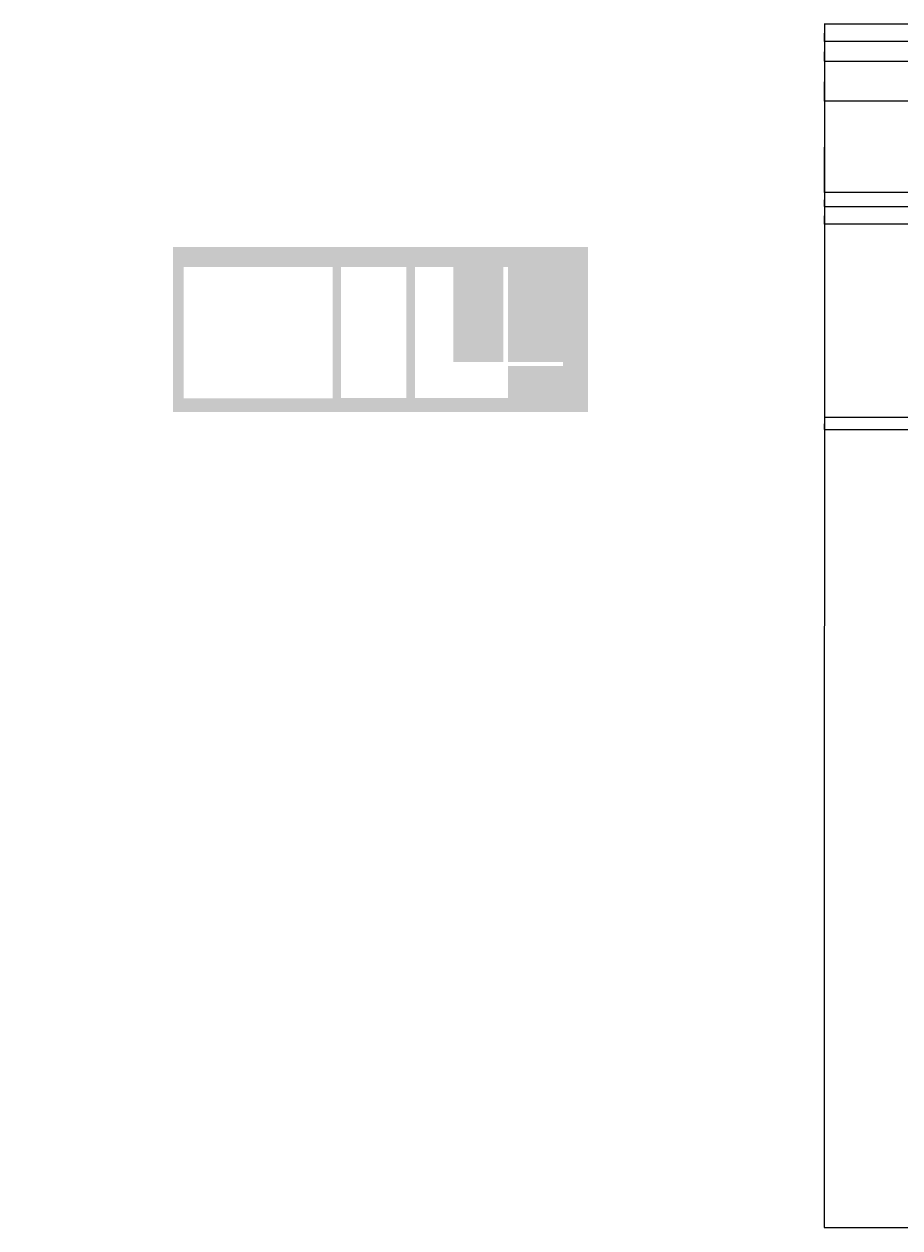
# Model space of a CAD drawing. Units: feet. Extents: x 1141 to 2858, y 751 to 1654.
# Tile 1 of 13: x 1141 to 1718, y 806 to 1599. Entities that reach past the tile are written whole.
import ezdxf

# ---------------------------------------------------------------- set-up
doc = ezdxf.new("R2010")
doc.units = ezdxf.units.FT
doc.layers.add('A-ANNO-DIMS', color=2, linetype='Continuous', lineweight=18)
doc.layers.add('A-ELEV-PATT', color=8, linetype='Continuous', lineweight=13)
doc.styles.get("Standard").update_dxf_attribs({"font": 'arial.ttf'})
doc.dimstyles.get("Standard").update_dxf_attribs({"dimtxt": 0.18, "dimasz": 0.18, "dimexe": 0.18, "dimexo": 0.0625, "dimgap": 0.09, "dimtad": 0, "dimtih": 1, "dimtoh": 1, "dimdec": 1, "dimzin": 0, "dimdsep": 46, "dimlunit": 3, "dimtxsty": 'Standard', "dimcen": 0.09, "dimadec": 0, "dimazin": 0, "dimtfac": 1, "dimtdec": 1, "dimtofl": 0, "dimtmove": 0, "dimatfit": 3, "dimfxl": 1, "dimtolj": 1, "dimtzin": 0, "dimarcsym": 0})

# ---------------------------------------------------------------- blocks, each defined once
blk = doc.blocks.new('*D24')
at = {"layer": 'A-ANNO-DIMS', "color": 0, "lineweight": -2, "transparency": 16777216}
for p, q in [((1725.97, 1599.45), (1668.14, 1599.45)), ((1668.32, 1599.27), (1668.32, 1202.86)), ((1668.32, 806.08), (1668.32, 1202.49)), ((1725.97, 805.9), (1668.14, 805.9))]:
    blk.add_line(p, q, dxfattribs=at)
at = {"layer": 'A-ANNO-DIMS', "color": 0, "transparency": 16777216}
for points in [[(1668.29, 1599.27), (1668.35, 1599.27), (1668.32, 1599.45)], [(1668.29, 806.08), (1668.35, 806.08), (1668.32, 805.9)]]:
    blk.add_solid(points, dxfattribs=at)
at = {"layer": 'Defpoints', "color": 0, "transparency": 16777216}
for p in [(1668.32, 1599.45), (1726.03, 1599.45), (1726.03, 805.9)]:
    blk.add_point(p, dxfattribs=at)
at = {"layer": 'A-ANNO-DIMS', "color": 0, "transparency": 16777216, "insert": (1668.32, 1202.68), "char_height": 0.18, "attachment_point": 5}
blk.add_mtext('\\A1;793.6', dxfattribs=at)
blk = doc.blocks.new('*D39')
at = {"layer": 'A-ANNO-DIMS', "color": 0, "lineweight": -2, "transparency": 16777216}
for p, q in [((2319.24, 1599.45), (1668.14, 1599.45)), ((1668.32, 1599.27), (1668.32, 1202.86)), ((1668.32, 806.08), (1668.32, 1202.49)), ((2319.24, 805.9), (1668.14, 805.9))]:
    blk.add_line(p, q, dxfattribs=at)
at = {"layer": 'A-ANNO-DIMS', "color": 0, "transparency": 16777216}
for points in [[(1668.29, 1599.27), (1668.35, 1599.27), (1668.32, 1599.45)], [(1668.29, 806.08), (1668.35, 806.08), (1668.32, 805.9)]]:
    blk.add_solid(points, dxfattribs=at)
at = {"layer": 'Defpoints', "color": 0, "transparency": 16777216}
for p in [(1668.32, 1599.45), (2319.3, 1599.45), (2319.3, 805.9)]:
    blk.add_point(p, dxfattribs=at)
at = {"layer": 'A-ANNO-DIMS', "color": 0, "transparency": 16777216, "insert": (1668.32, 1202.68), "char_height": 0.18, "attachment_point": 5}
blk.add_mtext('\\A1;793.6', dxfattribs=at)
blk = doc.blocks.new('*D48')
at = {"layer": 'A-ANNO-DIMS', "color": 0, "lineweight": -2, "transparency": 16777216}
for p, q in [((2330.82, 1479.03), (1668.14, 1479.03)), ((1668.32, 1478.85), (1668.32, 1473.42)), ((1668.32, 1467.63), (1668.32, 1473.06)), ((2319.24, 1467.45), (1668.14, 1467.45))]:
    blk.add_line(p, q, dxfattribs=at)
at = {"layer": 'A-ANNO-DIMS', "color": 0, "transparency": 16777216}
for points in [[(1668.29, 1478.85), (1668.35, 1478.85), (1668.32, 1479.03)], [(1668.29, 1467.63), (1668.35, 1467.63), (1668.32, 1467.45)]]:
    blk.add_solid(points, dxfattribs=at)
at = {"layer": 'Defpoints', "color": 0, "transparency": 16777216}
for p in [(1668.32, 1479.03), (2330.88, 1479.03), (2319.3, 1467.45)]:
    blk.add_point(p, dxfattribs=at)
at = {"layer": 'A-ANNO-DIMS', "color": 0, "transparency": 16777216, "insert": (1668.32, 1473.24), "char_height": 0.18, "attachment_point": 5}
blk.add_mtext('\\A1;11.58', dxfattribs=at)
blk = doc.blocks.new('*D49')
at = {"layer": 'A-ANNO-DIMS', "color": 0, "lineweight": -2, "transparency": 16777216}
for p, q in [((2347.45, 1488.33), (1668.14, 1488.33)), ((1668.32, 1488.15), (1668.32, 1483.86)), ((2330.82, 1479.03), (1668.14, 1479.03)), ((1668.32, 1479.21), (1668.32, 1483.5))]:
    blk.add_line(p, q, dxfattribs=at)
at = {"layer": 'A-ANNO-DIMS', "color": 0, "transparency": 16777216}
for points in [[(1668.29, 1488.15), (1668.35, 1488.15), (1668.32, 1488.33)], [(1668.29, 1479.21), (1668.35, 1479.21), (1668.32, 1479.03)]]:
    blk.add_solid(points, dxfattribs=at)
at = {"layer": 'Defpoints', "color": 0, "transparency": 16777216}
for p in [(1668.32, 1488.33), (2347.51, 1488.33), (2330.88, 1479.03)]:
    blk.add_point(p, dxfattribs=at)
at = {"layer": 'A-ANNO-DIMS', "color": 0, "transparency": 16777216, "insert": (1668.32, 1483.68), "char_height": 0.18, "attachment_point": 5}
blk.add_mtext('\\A1;9.293', dxfattribs=at)
blk = doc.blocks.new('*D50')
at = {"layer": 'A-ANNO-DIMS', "color": 0, "lineweight": -2, "transparency": 16777216}
for p, q in [((2356.58, 1548.54), (1668.14, 1548.54)), ((1668.32, 1548.36), (1668.32, 1518.62)), ((1668.32, 1488.51), (1668.32, 1518.25)), ((2347.45, 1488.33), (1668.14, 1488.33))]:
    blk.add_line(p, q, dxfattribs=at)
at = {"layer": 'A-ANNO-DIMS', "color": 0, "transparency": 16777216}
for points in [[(1668.29, 1548.36), (1668.35, 1548.36), (1668.32, 1548.54)], [(1668.29, 1488.51), (1668.35, 1488.51), (1668.32, 1488.33)]]:
    blk.add_solid(points, dxfattribs=at)
at = {"layer": 'Defpoints', "color": 0, "transparency": 16777216}
for p in [(1668.32, 1548.54), (2356.64, 1548.54), (2347.51, 1488.33)]:
    blk.add_point(p, dxfattribs=at)
at = {"layer": 'A-ANNO-DIMS', "color": 0, "transparency": 16777216, "insert": (1668.32, 1518.43), "char_height": 0.18, "attachment_point": 5}
blk.add_mtext('\\A1;60.22', dxfattribs=at)
blk = doc.blocks.new('*D51')
at = {"layer": 'A-ANNO-DIMS', "color": 0, "lineweight": -2, "transparency": 16777216}
for p, q in [((2347.45, 1574.77), (1668.14, 1574.77)), ((1668.32, 1574.59), (1668.32, 1561.84)), ((1668.32, 1548.72), (1668.32, 1561.47)), ((2356.58, 1548.54), (1668.14, 1548.54))]:
    blk.add_line(p, q, dxfattribs=at)
at = {"layer": 'A-ANNO-DIMS', "color": 0, "transparency": 16777216}
for points in [[(1668.29, 1574.59), (1668.35, 1574.59), (1668.32, 1574.77)], [(1668.29, 1548.72), (1668.35, 1548.72), (1668.32, 1548.54)]]:
    blk.add_solid(points, dxfattribs=at)
at = {"layer": 'Defpoints', "color": 0, "transparency": 16777216}
for p in [(1668.32, 1574.77), (2347.51, 1574.77), (2356.64, 1548.54)]:
    blk.add_point(p, dxfattribs=at)
at = {"layer": 'A-ANNO-DIMS', "color": 0, "transparency": 16777216, "insert": (1668.32, 1561.66), "char_height": 0.18, "attachment_point": 5}
blk.add_mtext('\\A1;26.23', dxfattribs=at)
blk = doc.blocks.new('*D52')
at = {"layer": 'A-ANNO-DIMS', "color": 0, "lineweight": -2, "transparency": 16777216}
for p, q in [((2330.82, 1587.87), (1668.14, 1587.87)), ((1668.32, 1587.69), (1668.32, 1581.5)), ((1668.32, 1574.95), (1668.32, 1581.14)), ((2347.45, 1574.77), (1668.14, 1574.77))]:
    blk.add_line(p, q, dxfattribs=at)
at = {"layer": 'A-ANNO-DIMS', "color": 0, "transparency": 16777216}
for points in [[(1668.29, 1587.69), (1668.35, 1587.69), (1668.32, 1587.87)], [(1668.29, 1574.95), (1668.35, 1574.95), (1668.32, 1574.77)]]:
    blk.add_solid(points, dxfattribs=at)
at = {"layer": 'Defpoints', "color": 0, "transparency": 16777216}
for p in [(1668.32, 1587.87), (2330.88, 1587.87), (2347.51, 1574.77)]:
    blk.add_point(p, dxfattribs=at)
at = {"layer": 'A-ANNO-DIMS', "color": 0, "transparency": 16777216, "insert": (1668.32, 1581.32), "char_height": 0.18, "attachment_point": 5}
blk.add_mtext('\\A1;13.102', dxfattribs=at)
blk = doc.blocks.new('*D53')
at = {"layer": 'A-ANNO-DIMS', "color": 0, "lineweight": -2, "transparency": 16777216}
for p, q in [((2319.24, 1599.45), (1668.14, 1599.45)), ((1668.32, 1599.27), (1668.32, 1593.84)), ((2330.82, 1587.87), (1668.14, 1587.87)), ((1668.32, 1588.05), (1668.32, 1593.48))]:
    blk.add_line(p, q, dxfattribs=at)
at = {"layer": 'A-ANNO-DIMS', "color": 0, "transparency": 16777216}
for points in [[(1668.29, 1599.27), (1668.35, 1599.27), (1668.32, 1599.45)], [(1668.29, 1588.05), (1668.35, 1588.05), (1668.32, 1587.87)]]:
    blk.add_solid(points, dxfattribs=at)
at = {"layer": 'Defpoints', "color": 0, "transparency": 16777216}
for p in [(1668.32, 1599.45), (2319.3, 1599.45), (2330.88, 1587.87)]:
    blk.add_point(p, dxfattribs=at)
at = {"layer": 'A-ANNO-DIMS', "color": 0, "transparency": 16777216, "insert": (1668.32, 1593.66), "char_height": 0.18, "attachment_point": 5}
blk.add_mtext('\\A1;11.58', dxfattribs=at)
blk = doc.blocks.new('*D54')
at = {"layer": 'A-ANNO-DIMS', "color": 0, "lineweight": -2, "transparency": 16777216}
for p, q in [((2327.22, 1340.05), (1668.14, 1340.05)), ((1668.32, 1339.87), (1668.32, 1336.24)), ((1668.32, 1332.24), (1668.32, 1335.88)), ((2319.24, 1332.06), (1668.14, 1332.06))]:
    blk.add_line(p, q, dxfattribs=at)
at = {"layer": 'A-ANNO-DIMS', "color": 0, "transparency": 16777216}
for points in [[(1668.29, 1339.87), (1668.35, 1339.87), (1668.32, 1340.05)], [(1668.29, 1332.24), (1668.35, 1332.24), (1668.32, 1332.06)]]:
    blk.add_solid(points, dxfattribs=at)
at = {"layer": 'Defpoints', "color": 0, "transparency": 16777216}
for p in [(1668.32, 1340.05), (2327.29, 1340.05), (2319.3, 1332.06)]:
    blk.add_point(p, dxfattribs=at)
at = {"layer": 'A-ANNO-DIMS', "color": 0, "transparency": 16777216, "insert": (1668.32, 1336.06), "char_height": 0.18, "attachment_point": 5}
blk.add_mtext('\\A1;7.986', dxfattribs=at)

msp = doc.modelspace()

# ---------------------------------------------------------------- hatches: boundary and pattern name
at = {"layer": 'A-ELEV-PATT'}
h = msp.add_hatch(color=256, dxfattribs=at)
h.dxf.hatch_style = 1
h.paths.add_polyline_path([(1219.3173, 1456.0789), (1140.7487, 1456.0789), (1156.2318, 1444.9949), (1219.3173, 1444.9949)], flags=0)
h.paths.add_polyline_path([(1156.2318, 1444.9949), (1140.7487, 1456.0789), (1140.7487, 1340.0506), (1156.2318, 1340.0506)], flags=0)
h.paths.add_polyline_path([(1156.2318, 1309.6069), (1187.7746, 1309.6069), (1187.7746, 1242.2735), (1219.3173, 1242.2735), (1219.3173, 1241.454), (1187.7746, 1241.454), (1187.7746, 1204.6626), (1186.8597, 1204.6626), (1186.8597, 1241.454), (1156.2318, 1241.454), (1156.2318, 1242.2735)], flags=0)
h.paths.add_polyline_path([(2109.4211, 1049.9149), (2030.8524, 1049.9149), (2030.8524, 1038.831), (2093.938, 1038.831), (2093.938, 933.8867), (2109.4211, 933.8867)], flags=0)
h.paths.add_polyline_path([(2109.4211, 1185.3029), (2030.8524, 1185.3029), (2030.8524, 1174.219), (2093.938, 1174.219), (2093.938, 1069.2747), (2109.4211, 1069.2747)])
h.paths.add_polyline_path([(1812.5866, 1320.6909), (1734.0179, 1320.6909), (1749.501, 1309.6069), (1812.5866, 1309.6069)])
h.paths.add_polyline_path([(1749.501, 1309.6069), (1734.0179, 1320.6909), (1734.0179, 1204.6626), (1749.501, 1204.6626)])
h.paths.add_polyline_path([(1812.5866, 1456.0789), (1734.0179, 1456.0789), (1749.501, 1444.9949), (1812.5866, 1444.9949)])
h.paths.add_polyline_path([(2117.407, 1057.9008), (2022.8666, 1057.9008), (2022.8666, 925.9008), (2117.407, 925.9008)])
h.paths.add_polyline_path([(2030.8524, 933.8867), (2030.8524, 1049.9149), (2109.4211, 1049.9149), (2109.4211, 933.8867)], flags=16)
h.paths.add_polyline_path([(2062.3952, 933.8867), (2062.3952, 970.6781), (2030.8524, 970.6781), (2030.8524, 971.4975), (2062.3952, 971.4975), (2062.3952, 1038.831), (2063.3101, 1038.831), (2093.938, 1038.831), (2093.938, 970.6781), (2063.3101, 970.6781), (2063.3101, 933.8867)], flags=0)
h = msp.add_hatch(color=256, dxfattribs=at)
h.dxf.hatch_style = 1
h.paths.add_polyline_path([(1512.5575, 1452.4845), (1238.8835, 1452.4845), (1238.8835, 1343.645), (1245.9375, 1352.9376), (1245.9375, 1439.3822), (1344.0874, 1439.3822), (1344.0874, 1352.9376), (1349.6277, 1352.9376), (1349.6277, 1439.3822), (1392.6132, 1439.3822), (1392.6132, 1352.9376), (1398.5284, 1352.9376), (1398.5284, 1439.3822), (1423.6034, 1439.3822), (1423.6034, 1376.6436), (1456.7296, 1376.6436), (1456.7296, 1439.3822), (1459.7654, 1439.3822), (1459.7654, 1376.6436), (1495.9275, 1376.6436), (1495.9275, 1373.9873), (1459.7654, 1373.9873), (1459.7654, 1352.9376), (1456.7296, 1352.9376), (1344.0874, 1352.9376), (1344.0874, 1352.8393), (1245.8629, 1352.8393), (1238.8835, 1343.645), (1512.5575, 1343.645)])
h.paths.add_polyline_path([(1790.4043, 1033.2183), (1754.2423, 1033.2183), (1754.2423, 970.4796), (1790.4043, 970.4796)])
h.paths.add_polyline_path([(1826.5664, 1033.2183), (1793.4402, 1033.2183), (1793.4402, 970.4796), (1826.5664, 970.4796)])
h.paths.add_polyline_path([(1826.5664, 967.8234), (1793.4402, 967.8234), (1793.4402, 946.7736), (1826.5664, 946.7736)])
h.paths.add_polyline_path([(1790.4043, 967.8234), (1754.2423, 967.8234), (1754.2423, 946.7736), (1790.4043, 946.7736)])
h.paths.add_polyline_path([(2093.938, 1038.831), (2063.3101, 1038.831), (2063.3101, 971.4975), (2093.938, 971.4975)])
h.paths.add_polyline_path([(2062.3952, 1038.831), (2030.8524, 1038.831), (2030.8524, 971.4975), (2062.3952, 971.4975)])
h.paths.add_polyline_path([(2062.3952, 970.6781), (2030.8524, 970.6781), (2030.8524, 933.8867), (2062.3952, 933.8867)])
h.paths.add_polyline_path([(2093.938, 970.6781), (2063.3101, 970.6781), (2063.3101, 933.8867), (2093.938, 933.8867)])

# ---------------------------------------------------------------- dimensions: what is measured, and where the dimension line sits
at = {"layer": 'A-ANNO-DIMS'}
for base, p1, p2, override, picture, middle in [((1668.3207, 1599.4527), (1726.032, 805.9008), (1726.032, 1599.4527), {"dimdec": 1, "dimlfac": 1, "dimrnd": 0, "dimzin": 0, "dimdsep": 46, "dimlunit": 2}, '*D24', (1668.3207, 1202.6768)), ((1668.3207, 1599.4527), (2319.3013, 805.9008), (2319.3013, 1599.4527), {"dimdec": 1, "dimlfac": 1, "dimrnd": 0, "dimzin": 0, "dimdsep": 46, "dimlunit": 2}, '*D39', (1668.3207, 1202.6768)), ((1668.3207, 1599.4527), (2330.8815, 1587.8725), (2319.3013, 1599.4527), {"dimdec": 2, "dimlfac": 1, "dimrnd": 0, "dimzin": 0, "dimdsep": 46, "dimlunit": 2}, '*D53', (1668.3207, 1593.6626)), ((1668.3207, 1587.8725), (2347.5116, 1574.7702), (2330.8815, 1587.8725), {"dimdec": 3, "dimlfac": 1, "dimrnd": 0, "dimzin": 0, "dimdsep": 46, "dimlunit": 2}, '*D52', (1668.3207, 1581.3214)), ((1668.3207, 1574.7702), (2356.6424, 1548.5407), (2347.5116, 1574.7702), {"dimdec": 2, "dimlfac": 1, "dimrnd": 0, "dimzin": 0, "dimdsep": 46, "dimlunit": 2}, '*D51', (1668.3207, 1561.6555)), ((1668.3207, 1548.5407), (2347.5116, 1488.3255), (2356.6424, 1548.5407), {"dimdec": 2, "dimlfac": 1, "dimrnd": 0, "dimzin": 0, "dimdsep": 46, "dimlunit": 2}, '*D50', (1668.3207, 1518.4331)), ((1668.32065, 1488.32554), (2330.88152, 1479.03299), (2347.51155, 1488.32554), {"dimdec": 3, "dimlfac": 1, "dimrnd": 0, "dimzin": 0, "dimdsep": 46, "dimlunit": 2}, '*D49', (1668.32065, 1483.67926)), ((1668.3207, 1479.033), (2319.3013, 1467.4527), (2330.8815, 1479.033), {"dimdec": 2, "dimlfac": 1, "dimrnd": 0, "dimzin": 0, "dimdsep": 46, "dimlunit": 2}, '*D48', (1668.3207, 1473.2429)), ((1668.3207, 1340.0506), (2319.3013, 1332.0647), (2327.2871, 1340.0506), {"dimdec": 3, "dimlfac": 1, "dimrnd": 0, "dimzin": 0, "dimdsep": 46, "dimlunit": 2}, '*D54', (1668.3207, 1336.0577))]:
    dim = msp.add_linear_dim(base=base, p1=p1, p2=p2, angle=90, dimstyle='Standard', override=override, dxfattribs=at)
    dim.commit()
    dim.dimension.update_dxf_attribs({"geometry": picture, "text_midpoint": middle})

doc.saveas('drawing.dxf')
